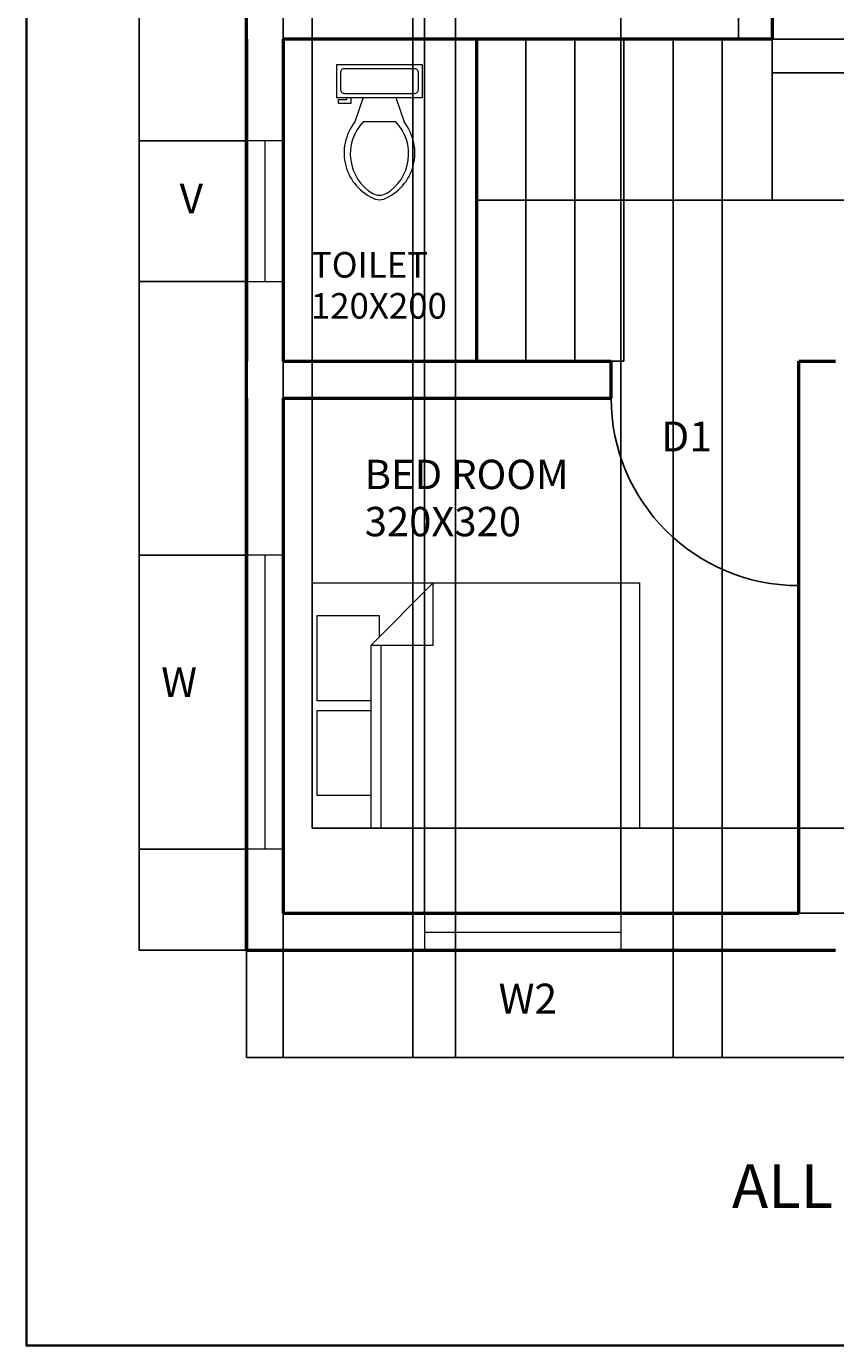
# Model space of a CAD drawing. Units: centimetres. Extents: x 2050 to 3144, y 831 to 2296.
# Tile 1 of 7: x 2050 to 2553, y 831 to 1650. Entities that reach past the tile are written whole.
import ezdxf

# ---------------------------------------------------------------- set-up
doc = ezdxf.new("R2010")
doc.units = ezdxf.units.CM
for name, color, linetype, lineweight in [('A-ANNO-DIMS', 2, 'Continuous', 18), ('A-ANNO-TEXT', 7, 'Continuous', 18), ('A-ANNO-TTLB', 7, 'Continuous', 35), ('A-AREA-IDEN', 7, 'Continuous', 25), ('A-DOOR', 3, 'Continuous', 25), ('A-FLOR-FIXT', 8, 'Continuous', 18), ('A-FLOR-STRS', 7, 'Continuous', 25), ('A-FURN', 8, 'Continuous', 18), ('A-GLAZ', 4, 'Continuous', 18), ('A-WALL', 7, 'Continuous', 50)]:
    doc.layers.add(name, color=color, linetype=linetype, lineweight=lineweight)
doc.styles.get("Standard").update_dxf_attribs({"font": 'arial.ttf'})
doc.dimstyles.get("Standard").update_dxf_attribs({"dimtxt": 0.18, "dimasz": 0.18, "dimexe": 0.18, "dimexo": 0.0625, "dimgap": 0.09, "dimtad": 0, "dimtih": 1, "dimtoh": 1, "dimdec": 4, "dimzin": 0, "dimdsep": 46, "dimtxsty": 'Standard', "dimcen": 0.09, "dimadec": 0, "dimazin": 0, "dimtfac": 1, "dimtdec": 4, "dimtofl": 0, "dimtmove": 0, "dimatfit": 3, "dimfxl": 1, "dimtolj": 1, "dimtzin": 0, "dimarcsym": 0})

# ---------------------------------------------------------------- blocks, each defined once
blk = doc.blocks.new('Toilet - top')
for p, q in [((9.5, -6), (9.5, -2)), ((-10, -8.5), (-8, -8.5)), ((-10, -9.5), (-10, -8.5)), ((-7, -9.5), (-10, -9.5)), ((-8, -8.5), (-8, -8)), ((-7, -8), (-7, -9.5)), ((-4, -8), (-6, -14)), ((4, -8), (6, -14)), ((4, -14), (-4, -14))]:
    blk.add_line(p, q)
blk.add_lwpolyline([(10.5, -8), (10.5, 0), (-10.5, 0), (-10.5, -8)], close=True)
for points in [[(-9.5, -2), (-9.5, -6)], [(8.5, -1), (-8.5, -1)], [(-8.5, -7), (8.5, -7)]]:
    blk.add_lwpolyline(points)
for centre, radius, start, end in [((-8.62, -1.88), 0.884, 81.8699, 188.1301), ((8.62, -1.88), 0.884, 351.8699, 98.1301), ((-8.62, -6.12), 0.884, 171.8699, 278.1301), ((8.62, -6.12), 0.884, 261.8699, 8.1301), ((3.52, -21.58), 12.17, 141.4691, 247.9714), ((4.2, -21.82), 11.33, 136.3677, 238.9468), ((-3.52, -21.58), 12.17, 292.0284, 38.5307), ((-4.2, -21.82), 11.33, 301.053, 43.6321), ((0, -27.88), 4, 245.7318, 294.2682), ((0, -29), 4, 254.8605, 285.1395)]:
    blk.add_arc(centre, radius, start, end)
blk = doc.blocks.new('Bed - Queen')
for p, q in [((0, -80.00003), (0, 0)), ((0, 0), (59.99999, 0)), ((59.99999, 0), (59.99999, -80.00003)), ((7.99999, -1.2), (28.79998, -1.2)), ((7.99999, -14.4), (7.99999, -1.2)), ((28.79998, -1.2), (28.79998, -14.4)), ((31.19999, -1.2), (51.99999, -1.2)), ((31.19999, -14.4), (31.19999, -1.2)), ((51.99999, -1.2), (51.99999, -16.4)), ((0, -14.4), (44.8, -14.4)), ((59.99999, -29.6), (44.8, -14.4)), ((44.8, -14.4), (44.8, -29.6)), ((44.8, -16.8), (0, -16.8)), ((51.99999, -16.4), (46.79936, -16.4)), ((44.8, -29.6), (59.99999, -29.6)), ((59.99999, -80.00003), (0, -80.00003))]:
    blk.add_line(p, q)
blk = doc.blocks.new('DOOR-D1-1165')
blk.add_line((116.51, 0), (116.51, 139.37))
blk.add_arc((116.51, 116.51), 116.51, 180, 270)
blk = doc.blocks.new('*D15')
at = {"layer": 'A-ANNO-DIMS', "color": 0, "lineweight": -2, "transparency": 16777216}
for p, q in [((2513.3, 1781.4), (2492.28, 1781.4)), ((2492.46, 1781.22), (2492.46, 1711.9)), ((2492.46, 1642.21), (2492.46, 1711.53)), ((2513.3, 1642.03), (2492.28, 1642.03))]:
    blk.add_line(p, q, dxfattribs=at)
at = {"layer": 'A-ANNO-DIMS', "color": 0, "transparency": 16777216}
for points in [[(2492.43, 1781.22), (2492.49, 1781.22), (2492.46, 1781.4)], [(2492.43, 1642.21), (2492.49, 1642.21), (2492.46, 1642.03)]]:
    blk.add_solid(points, dxfattribs=at)
at = {"layer": 'Defpoints', "color": 0, "transparency": 16777216}
for p in [(2513.36, 1781.4), (2492.46, 1642.03), (2513.36, 1642.03)]:
    blk.add_point(p, dxfattribs=at)
at = {"layer": 'A-ANNO-DIMS', "color": 0, "transparency": 16777216, "insert": (2492.46, 1711.72), "char_height": 0.18, "attachment_point": 5}
blk.add_mtext('\\A1;DOOR D1 139 TYP.', dxfattribs=at)
blk = doc.blocks.new('*D16')
at = {"layer": 'A-ANNO-DIMS', "color": 0, "lineweight": -2, "transparency": 16777216}
for p, q in [((2513.36, 1641.97), (2513.36, 1620.95)), ((2629.87, 1641.97), (2629.87, 1620.95)), ((2513.54, 1621.13), (2571.02, 1621.13)), ((2629.69, 1621.13), (2572.2, 1621.13))]:
    blk.add_line(p, q, dxfattribs=at)
at = {"layer": 'A-ANNO-DIMS', "color": 0, "transparency": 16777216}
for points in [[(2513.54, 1621.16), (2513.54, 1621.1), (2513.36, 1621.13)], [(2629.69, 1621.16), (2629.69, 1621.1), (2629.87, 1621.13)]]:
    blk.add_solid(points, dxfattribs=at)
at = {"layer": 'Defpoints', "color": 0, "transparency": 16777216}
for p in [(2513.36, 1642.03), (2629.87, 1642.03), (2629.87, 1621.13)]:
    blk.add_point(p, dxfattribs=at)
at = {"layer": 'A-ANNO-DIMS', "color": 0, "transparency": 16777216, "insert": (2571.61, 1621.13), "char_height": 0.18, "attachment_point": 5}
blk.add_mtext('\\A1;117 TYP.', dxfattribs=at)
blk = doc.blocks.new('*D31')
at = {"layer": 'A-ANNO-DIMS', "color": 0, "lineweight": -2, "transparency": 16777216}
for p, q in [((2187.01, 1076.25), (2187.01, 1009.53)), ((2975.59, 1076.25), (2975.59, 1009.53)), ((2187.19, 1009.71), (2580.9, 1009.71)), ((2975.41, 1009.71), (2581.69, 1009.71))]:
    blk.add_line(p, q, dxfattribs=at)
at = {"layer": 'A-ANNO-DIMS', "color": 0, "transparency": 16777216}
for points in [[(2187.19, 1009.74), (2187.19, 1009.68), (2187.01, 1009.71)], [(2975.41, 1009.74), (2975.41, 1009.68), (2975.59, 1009.71)]]:
    blk.add_solid(points, dxfattribs=at)
at = {"layer": 'Defpoints', "color": 0, "transparency": 16777216}
for p in [(2187.01, 1076.31), (2975.59, 1076.31), (2975.59, 1009.71)]:
    blk.add_point(p, dxfattribs=at)
at = {"layer": 'A-ANNO-DIMS', "color": 0, "transparency": 16777216, "insert": (2581.3, 1009.71), "char_height": 0.18, "attachment_point": 5}
blk.add_mtext('\\A1;788.6', dxfattribs=at)
blk = doc.blocks.new('*D32')
at = {"layer": 'A-ANNO-DIMS', "color": 0, "lineweight": -2, "transparency": 16777216}
for p, q in [((2186.94, 2087.75), (2120.23, 2087.75)), ((2120.41, 2087.57), (2120.41, 1582.22)), ((2120.41, 1076.49), (2120.41, 1581.85)), ((2186.94, 1076.31), (2120.23, 1076.31))]:
    blk.add_line(p, q, dxfattribs=at)
at = {"layer": 'A-ANNO-DIMS', "color": 0, "transparency": 16777216}
for points in [[(2120.38, 2087.57), (2120.44, 2087.57), (2120.41, 2087.75)], [(2120.38, 1076.49), (2120.44, 1076.49), (2120.41, 1076.31)]]:
    blk.add_solid(points, dxfattribs=at)
at = {"layer": 'Defpoints', "color": 0, "transparency": 16777216}
for p in [(2120.41, 2087.75), (2187.01, 2087.75), (2187.01, 1076.31)]:
    blk.add_point(p, dxfattribs=at)
at = {"layer": 'A-ANNO-DIMS', "color": 0, "transparency": 16777216, "insert": (2120.41, 1582.03), "char_height": 0.18, "attachment_point": 5}
blk.add_mtext('\\A1;1011.4', dxfattribs=at)
blk = doc.blocks.new('*D38')
at = {"layer": 'A-ANNO-DIMS', "color": 0, "lineweight": -2, "transparency": 16777216}
for p, q in [((2186.94, 1139.08), (2120.23, 1139.08)), ((2120.41, 1138.9), (2120.41, 1107.88)), ((2120.41, 1076.49), (2120.41, 1107.52)), ((2186.94, 1076.31), (2120.23, 1076.31))]:
    blk.add_line(p, q, dxfattribs=at)
at = {"layer": 'A-ANNO-DIMS', "color": 0, "transparency": 16777216}
for points in [[(2120.38, 1138.9), (2120.44, 1138.9), (2120.41, 1139.08)], [(2120.38, 1076.49), (2120.44, 1076.49), (2120.41, 1076.31)]]:
    blk.add_solid(points, dxfattribs=at)
at = {"layer": 'Defpoints', "color": 0, "transparency": 16777216}
for p in [(2120.41, 1139.08), (2187.01, 1139.08), (2187.01, 1076.31)]:
    blk.add_point(p, dxfattribs=at)
at = {"layer": 'A-ANNO-DIMS', "color": 0, "transparency": 16777216, "insert": (2120.41, 1107.7), "char_height": 0.18, "attachment_point": 5}
blk.add_mtext('\\A1;62.77', dxfattribs=at)
blk = doc.blocks.new('*D39')
at = {"layer": 'A-ANNO-DIMS', "color": 0, "lineweight": -2, "transparency": 16777216}
for p, q in [((2186.94, 1321.51), (2120.23, 1321.51)), ((2120.41, 1321.33), (2120.41, 1230.48)), ((2120.41, 1139.26), (2120.41, 1230.12)), ((2186.94, 1139.08), (2120.23, 1139.08))]:
    blk.add_line(p, q, dxfattribs=at)
at = {"layer": 'A-ANNO-DIMS', "color": 0, "transparency": 16777216}
for points in [[(2120.38, 1321.33), (2120.44, 1321.33), (2120.41, 1321.51)], [(2120.38, 1139.26), (2120.44, 1139.26), (2120.41, 1139.08)]]:
    blk.add_solid(points, dxfattribs=at)
at = {"layer": 'Defpoints', "color": 0, "transparency": 16777216}
for p in [(2120.41, 1321.51), (2187.01, 1321.51), (2187.01, 1139.08)]:
    blk.add_point(p, dxfattribs=at)
at = {"layer": 'A-ANNO-DIMS', "color": 0, "transparency": 16777216, "insert": (2120.41, 1230.3), "char_height": 0.18, "attachment_point": 5}
blk.add_mtext('\\A1;182.43', dxfattribs=at)
blk = doc.blocks.new('*D40')
at = {"layer": 'A-ANNO-DIMS', "color": 0, "lineweight": -2, "transparency": 16777216}
for p, q in [((2186.94, 1491.53), (2120.23, 1491.53)), ((2120.41, 1491.35), (2120.41, 1406.7)), ((2120.41, 1321.69), (2120.41, 1406.34)), ((2186.94, 1321.51), (2120.23, 1321.51))]:
    blk.add_line(p, q, dxfattribs=at)
at = {"layer": 'A-ANNO-DIMS', "color": 0, "transparency": 16777216}
for points in [[(2120.38, 1491.35), (2120.44, 1491.35), (2120.41, 1491.53)], [(2120.38, 1321.69), (2120.44, 1321.69), (2120.41, 1321.51)]]:
    blk.add_solid(points, dxfattribs=at)
at = {"layer": 'Defpoints', "color": 0, "transparency": 16777216}
for p in [(2120.41, 1491.53), (2187.01, 1491.53), (2187.01, 1321.51)]:
    blk.add_point(p, dxfattribs=at)
at = {"layer": 'A-ANNO-DIMS', "color": 0, "transparency": 16777216, "insert": (2120.41, 1406.52), "char_height": 0.18, "attachment_point": 5}
blk.add_mtext('\\A1;170.02', dxfattribs=at)
blk = doc.blocks.new('*D41')
at = {"layer": 'A-ANNO-DIMS', "color": 0, "lineweight": -2, "transparency": 16777216}
for p, q in [((2186.94, 1578.89), (2120.23, 1578.89)), ((2120.41, 1578.71), (2120.41, 1535.39)), ((2120.41, 1491.71), (2120.41, 1535.03)), ((2186.94, 1491.53), (2120.23, 1491.53))]:
    blk.add_line(p, q, dxfattribs=at)
at = {"layer": 'A-ANNO-DIMS', "color": 0, "transparency": 16777216}
for points in [[(2120.38, 1578.71), (2120.44, 1578.71), (2120.41, 1578.89)], [(2120.38, 1491.71), (2120.44, 1491.71), (2120.41, 1491.53)]]:
    blk.add_solid(points, dxfattribs=at)
at = {"layer": 'Defpoints', "color": 0, "transparency": 16777216}
for p in [(2120.41, 1578.89), (2187.01, 1578.89), (2187.01, 1491.53)]:
    blk.add_point(p, dxfattribs=at)
at = {"layer": 'A-ANNO-DIMS', "color": 0, "transparency": 16777216, "insert": (2120.41, 1535.21), "char_height": 0.18, "attachment_point": 5}
blk.add_mtext('\\A1;87.36', dxfattribs=at)
blk = doc.blocks.new('*D42')
at = {"layer": 'A-ANNO-DIMS', "color": 0, "lineweight": -2, "transparency": 16777216}
for p, q in [((2186.94, 1742.97), (2120.23, 1742.97)), ((2120.41, 1742.79), (2120.41, 1661.12)), ((2120.41, 1579.07), (2120.41, 1660.75)), ((2186.94, 1578.89), (2120.23, 1578.89))]:
    blk.add_line(p, q, dxfattribs=at)
at = {"layer": 'A-ANNO-DIMS', "color": 0, "transparency": 16777216}
for points in [[(2120.38, 1742.79), (2120.44, 1742.79), (2120.41, 1742.97)], [(2120.38, 1579.07), (2120.44, 1579.07), (2120.41, 1578.89)]]:
    blk.add_solid(points, dxfattribs=at)
at = {"layer": 'Defpoints', "color": 0, "transparency": 16777216}
for p in [(2120.41, 1742.97), (2187.01, 1742.97), (2187.01, 1578.89)]:
    blk.add_point(p, dxfattribs=at)
at = {"layer": 'A-ANNO-DIMS', "color": 0, "transparency": 16777216, "insert": (2120.41, 1660.93), "char_height": 0.18, "attachment_point": 5}
blk.add_mtext('\\A1;164.08', dxfattribs=at)
blk = doc.blocks.new('*D47')
at = {"layer": 'A-ANNO-DIMS', "color": 0, "lineweight": -2, "transparency": 16777216}
for p, q in [((2209.87, 1099.24), (2209.87, 2154.53)), ((2210.05, 2154.35), (2253.35, 2154.35)), ((2297.29, 2154.35), (2253.99, 2154.35)), ((2297.47, 1099.24), (2297.47, 2154.53))]:
    blk.add_line(p, q, dxfattribs=at)
at = {"layer": 'A-ANNO-DIMS', "color": 0, "transparency": 16777216}
for points in [[(2210.05, 2154.38), (2210.05, 2154.32), (2209.87, 2154.35)], [(2297.29, 2154.38), (2297.29, 2154.32), (2297.47, 2154.35)]]:
    blk.add_solid(points, dxfattribs=at)
at = {"layer": 'Defpoints', "color": 0, "transparency": 16777216}
for p in [(2297.47, 2154.35), (2209.87, 1099.17), (2297.47, 1099.17)]:
    blk.add_point(p, dxfattribs=at)
at = {"layer": 'A-ANNO-DIMS', "color": 0, "transparency": 16777216, "insert": (2253.67, 2154.35), "char_height": 0.18, "attachment_point": 5}
blk.add_mtext('\\A1;87.6', dxfattribs=at)
blk = doc.blocks.new('*D51')
at = {"layer": 'A-ANNO-DIMS', "color": 0, "lineweight": -2, "transparency": 16777216}
for p, q in [((2451.79, 1541.97), (2451.79, 1009.53)), ((2482.27, 1541.97), (2482.27, 1009.53)), ((2451.97, 1009.71), (2466.63, 1009.71)), ((2482.09, 1009.71), (2467.42, 1009.71))]:
    blk.add_line(p, q, dxfattribs=at)
at = {"layer": 'A-ANNO-DIMS', "color": 0, "transparency": 16777216}
for points in [[(2451.97, 1009.74), (2451.97, 1009.68), (2451.79, 1009.71)], [(2482.09, 1009.74), (2482.09, 1009.68), (2482.27, 1009.71)]]:
    blk.add_solid(points, dxfattribs=at)
at = {"layer": 'Defpoints', "color": 0, "transparency": 16777216}
for p in [(2451.79, 1542.03), (2482.27, 1542.03), (2482.27, 1009.71)]:
    blk.add_point(p, dxfattribs=at)
at = {"layer": 'A-ANNO-DIMS', "color": 0, "transparency": 16777216, "insert": (2467.03, 1009.71), "char_height": 0.18, "attachment_point": 5}
blk.add_mtext('\\A1;30.48', dxfattribs=at)
blk = doc.blocks.new('*D52')
at = {"layer": 'A-ANNO-DIMS', "color": 0, "lineweight": -2, "transparency": 16777216}
for p, q in [((2513.42, 1642.03), (3042.37, 1642.03)), ((3042.19, 1641.85), (3042.19, 1592.22)), ((3042.19, 1542.21), (3042.19, 1591.85)), ((2513.42, 1542.03), (3042.37, 1542.03))]:
    blk.add_line(p, q, dxfattribs=at)
at = {"layer": 'A-ANNO-DIMS', "color": 0, "transparency": 16777216}
for points in [[(3042.16, 1641.85), (3042.22, 1641.85), (3042.19, 1642.03)], [(3042.16, 1542.21), (3042.22, 1542.21), (3042.19, 1542.03)]]:
    blk.add_solid(points, dxfattribs=at)
at = {"layer": 'Defpoints', "color": 0, "transparency": 16777216}
for p in [(2513.36, 1642.03), (3042.19, 1642.03), (2513.36, 1542.03)]:
    blk.add_point(p, dxfattribs=at)
at = {"layer": 'A-ANNO-DIMS', "color": 0, "transparency": 16777216, "insert": (3042.19, 1592.03), "char_height": 0.18, "attachment_point": 5}
blk.add_mtext('\\A1;100', dxfattribs=at)
blk = doc.blocks.new('*D53')
at = {"layer": 'A-ANNO-DIMS', "color": 0, "lineweight": -2, "transparency": 16777216}
for p, q in [((2209.87, 1664.83), (2209.87, 1009.53)), ((2290.25, 1664.83), (2290.25, 1009.53)), ((2210.05, 1009.71), (2249.67, 1009.71)), ((2290.07, 1009.71), (2250.45, 1009.71))]:
    blk.add_line(p, q, dxfattribs=at)
at = {"layer": 'A-ANNO-DIMS', "color": 0, "transparency": 16777216}
for points in [[(2210.05, 1009.74), (2210.05, 1009.68), (2209.87, 1009.71)], [(2290.07, 1009.74), (2290.07, 1009.68), (2290.25, 1009.71)]]:
    blk.add_solid(points, dxfattribs=at)
at = {"layer": 'Defpoints', "color": 0, "transparency": 16777216}
for p in [(2209.87, 1664.89), (2290.25, 1664.89), (2290.25, 1009.71)]:
    blk.add_point(p, dxfattribs=at)
at = {"layer": 'A-ANNO-DIMS', "color": 0, "transparency": 16777216, "insert": (2250.06, 1009.71), "char_height": 0.18, "attachment_point": 5}
blk.add_mtext('\\A1;80.39', dxfattribs=at)
blk = doc.blocks.new('*D63')
at = {"layer": 'A-ANNO-DIMS', "color": 0, "lineweight": -2, "transparency": 16777216}
for p, q in [((2297.47, 1099.24), (2297.47, 2154.53)), ((2297.65, 2154.35), (2357.98, 2154.35)), ((2419.21, 2154.35), (2358.89, 2154.35)), ((2419.39, 1099.24), (2419.39, 2154.53))]:
    blk.add_line(p, q, dxfattribs=at)
at = {"layer": 'A-ANNO-DIMS', "color": 0, "transparency": 16777216}
for points in [[(2297.65, 2154.38), (2297.65, 2154.32), (2297.47, 2154.35)], [(2419.21, 2154.38), (2419.21, 2154.32), (2419.39, 2154.35)]]:
    blk.add_solid(points, dxfattribs=at)
at = {"layer": 'Defpoints', "color": 0, "transparency": 16777216}
for p in [(2419.39, 2154.35), (2297.47, 1099.17), (2419.39, 1099.17)]:
    blk.add_point(p, dxfattribs=at)
at = {"layer": 'A-ANNO-DIMS', "color": 0, "transparency": 16777216, "insert": (2358.43, 2154.35), "char_height": 0.18, "attachment_point": 5}
blk.add_mtext('\\A1;121.92', dxfattribs=at)
blk = doc.blocks.new('*D66')
at = {"layer": 'A-ANNO-DIMS', "color": 0, "lineweight": -2, "transparency": 16777216}
for p, q in [((2209.87, 1139.14), (2209.87, 2154.53)), ((2210.05, 2154.35), (2218.38, 2154.35)), ((2227.62, 2154.35), (2219.29, 2154.35)), ((2227.8, 1152.03), (2227.8, 2154.53))]:
    blk.add_line(p, q, dxfattribs=at)
at = {"layer": 'A-ANNO-DIMS', "color": 0, "transparency": 16777216}
for points in [[(2210.05, 2154.38), (2210.05, 2154.32), (2209.87, 2154.35)], [(2227.62, 2154.38), (2227.62, 2154.32), (2227.8, 2154.35)]]:
    blk.add_solid(points, dxfattribs=at)
at = {"layer": 'Defpoints', "color": 0, "transparency": 16777216}
for p in [(2227.8, 2154.35), (2227.8, 1151.97), (2209.87, 1139.08)]:
    blk.add_point(p, dxfattribs=at)
at = {"layer": 'A-ANNO-DIMS', "color": 0, "transparency": 16777216, "insert": (2218.83, 2154.35), "char_height": 0.18, "attachment_point": 5}
blk.add_mtext('\\A1;17.933', dxfattribs=at)
blk = doc.blocks.new('*D67')
at = {"layer": 'A-ANNO-DIMS', "color": 0, "lineweight": -2, "transparency": 16777216}
for p, q in [((2227.86, 1151.97), (3042.37, 1151.97)), ((3042.19, 1151.79), (3042.19, 1125.75)), ((3042.19, 1099.35), (3042.19, 1125.39)), ((2209.93, 1099.17), (3042.37, 1099.17))]:
    blk.add_line(p, q, dxfattribs=at)
at = {"layer": 'A-ANNO-DIMS', "color": 0, "transparency": 16777216}
for points in [[(3042.16, 1151.79), (3042.22, 1151.79), (3042.19, 1151.97)], [(3042.16, 1099.35), (3042.22, 1099.35), (3042.19, 1099.17)]]:
    blk.add_solid(points, dxfattribs=at)
at = {"layer": 'Defpoints', "color": 0, "transparency": 16777216}
for p in [(2227.8, 1151.97), (2209.87, 1099.17), (3042.19, 1099.17)]:
    blk.add_point(p, dxfattribs=at)
at = {"layer": 'A-ANNO-DIMS', "color": 0, "transparency": 16777216, "insert": (3042.19, 1125.57), "char_height": 0.18, "attachment_point": 5}
blk.add_mtext('\\A1;52.79', dxfattribs=at)
blk = doc.blocks.new('*D70')
at = {"layer": 'A-ANNO-DIMS', "color": 0, "lineweight": -2, "transparency": 16777216}
for p, q in [((2209.87, 2064.83), (2209.87, 1009.53)), ((2316.84, 2059.23), (2316.84, 1009.53)), ((2210.05, 1009.71), (2262.9, 1009.71)), ((2316.66, 1009.71), (2263.81, 1009.71))]:
    blk.add_line(p, q, dxfattribs=at)
at = {"layer": 'A-ANNO-DIMS', "color": 0, "transparency": 16777216}
for points in [[(2210.05, 1009.74), (2210.05, 1009.68), (2209.87, 1009.71)], [(2316.66, 1009.74), (2316.66, 1009.68), (2316.84, 1009.71)]]:
    blk.add_solid(points, dxfattribs=at)
at = {"layer": 'Defpoints', "color": 0, "transparency": 16777216}
for p in [(2209.87, 2064.89), (2316.84, 2059.29), (2316.84, 1009.71)]:
    blk.add_point(p, dxfattribs=at)
at = {"layer": 'A-ANNO-DIMS', "color": 0, "transparency": 16777216, "insert": (2263.35, 1009.71), "char_height": 0.18, "attachment_point": 5}
blk.add_mtext('\\A1;106.97', dxfattribs=at)

msp = doc.modelspace()

# ---------------------------------------------------------------- linework, layer by layer
at = {"layer": 'A-ANNO-TTLB'}
msp.add_lwpolyline([(2050.3641, 2295.8578), (3143.7558, 2295.8578), (3143.7558, 830.6902), (2050.3641, 830.6902)], close=True, dxfattribs=at)
at = {"layer": 'A-FLOR-STRS'}
for p, q in [((2360.3465, 1642.0348), (2360.3465, 1442.0348)), ((2390.8265, 1642.0348), (2390.8265, 1442.0348)), ((2421.3065, 1642.0348), (2421.3065, 1442.0348)), ((2451.7865, 1642.0348), (2451.7865, 1542.0348)), ((2482.2665, 1642.0348), (2482.2665, 1542.0348)), ((2513.3612, 1642.0348), (2513.3612, 1542.0348)), ((2513.3612, 1542.0348), (2329.8665, 1542.0348)), ((2413.3612, 1442.0348), (2421.3065, 1442.0348))]:
    msp.add_line(p, q, dxfattribs=at)
at = {"layer": 'A-GLAZ'}
for p, q in [((2209.8665, 1578.8921), (2187.0065, 1578.8921)), ((2198.4365, 1578.8921), (2198.4365, 1491.5301)), ((2187.0065, 1491.5301), (2209.8665, 1491.5301)), ((2209.8665, 1321.513), (2187.0065, 1321.513)), ((2198.4365, 1321.513), (2198.4365, 1139.0811)), ((2209.8665, 1139.0811), (2187.0065, 1139.0811)), ((2297.4733, 1099.1748), (2297.4733, 1076.3148)), ((2419.3933, 1099.1748), (2419.3933, 1076.3148)), ((2297.4733, 1087.4723), (2419.3933, 1087.4723))]:
    msp.add_line(p, q, dxfattribs=at)
at = {"layer": 'A-WALL'}
for p, q in [((2187.0065, 1076.3148), (2187.0065, 2087.7548)), ((2513.3612, 1664.8948), (2513.3612, 1642.0348)), ((2187.0065, 1642.0348), (2187.0065, 1442.0348)), ((2209.8665, 1642.0348), (2209.8665, 1442.0348)), ((2513.3612, 1642.0348), (2209.8665, 1642.0348)), ((2329.8665, 1642.0348), (2329.8665, 1442.0348)), ((2209.8665, 1442.0348), (2413.3612, 1442.0348)), ((2413.3612, 1419.1748), (2413.3612, 1442.0348)), ((2529.8665, 1099.1748), (2529.8665, 1442.0348)), ((2529.8665, 1442.0348), (2552.7265, 1442.0348)), ((2187.0065, 1419.1748), (2187.0065, 1076.3148)), ((2209.8665, 1419.1748), (2413.3612, 1419.1748)), ((2209.8665, 1419.1748), (2209.8665, 1099.1748)), ((2209.8665, 1099.1748), (2529.8665, 1099.1748)), ((2187.0065, 1076.3148), (2552.7265, 1076.3148))]:
    msp.add_line(p, q, dxfattribs=at)

# ---------------------------------------------------------------- block references
at = {"layer": 'A-DOOR', "extrusion": (0, 0, -1), "zscale": -1, "rotation": 180}
msp.add_blockref('DOOR-D1-1165', (-2513.361, 1781.4006), dxfattribs=at)
at = {"layer": 'A-DOOR'}
msp.add_blockref('DOOR-D1-1165', (2413.361, 1302.669), dxfattribs=at)
at = {"layer": 'A-FLOR-FIXT', "xscale": 2.54, "yscale": 2.54, "zscale": 2.54}
msp.add_blockref('Toilet - top', (2269.5685, 1626.163), dxfattribs=at)
at = {"layer": 'A-FURN', "xscale": 2.54, "yscale": 2.54, "zscale": 2.54, "rotation": 90}
msp.add_blockref('Bed - Queen', (2227.7996, 1151.9671), dxfattribs=at)

# ---------------------------------------------------------------- texts
at = {"layer": 'A-ANNO-TEXT'}
for s, height, p in [('V', 18.5959, (2145.4428, 1533.7818)), ('D1', 18.59595, (2444.4269, 1385.9903)), ('W', 18.5959, (2134.0485, 1233.4159)), ('W2', 18.59595, (2343.4962, 1036.8754)), ('ALL DIMENSION IN CENTIMETER', 27.192544, (2488.3592, 916.1363))]:
    msp.add_text(s, height=height, dxfattribs=at).set_placement(p)
at = {"layer": 'A-AREA-IDEN'}
for s, height, p in [('TOILET', 15.8597, (2226.9643, 1493.9662)), ('120X200', 15.8597, (2226.9643, 1468.489)), ('BED ROOM', 18.23402, (2260.3697, 1362.6011)), ('320X320', 18.23402, (2260.3697, 1333.3098))]:
    msp.add_text(s, height=height, dxfattribs=at).set_placement(p)

# ---------------------------------------------------------------- dimensions: what is measured, and where the dimension line sits
at = {"layer": 'A-ANNO-DIMS'}
for base, p1, p2, override, picture, middle in [((2297.4733, 2154.3548), (2209.8665, 1099.1748), (2297.4733, 1099.1748), {"dimdec": 1, "dimlfac": 1, "dimrnd": 0, "dimzin": 0, "dimdsep": 46, "dimlunit": 2}, '*D47', (2253.6699, 2154.3548)), ((2227.7996, 2154.3548), (2209.8665, 1139.0811), (2227.7996, 1151.9671), {"dimdec": 3, "dimlfac": 1, "dimrnd": 0, "dimzin": 0, "dimdsep": 46, "dimlunit": 2}, '*D66', (2218.8331, 2154.3548)), ((2419.3933, 2154.3548), (2297.4733, 1099.1748), (2419.3933, 1099.1748), {"dimdec": 2, "dimlfac": 1, "dimrnd": 0, "dimzin": 0, "dimdsep": 46, "dimlunit": 2}, '*D63', (2358.4333, 2154.3548)), ((2316.8368, 1009.7148), (2209.8665, 2064.8948), (2316.8368, 2059.2924), {"dimdec": 2, "dimlfac": 1, "dimrnd": 0, "dimzin": 0, "dimdsep": 46, "dimlunit": 2}, '*D70', (2263.3517, 1009.7148)), ((2290.2526, 1009.7148), (2209.8665, 1664.8948), (2290.2526, 1664.8948), {"dimdec": 2, "dimlfac": 1, "dimrnd": 0, "dimzin": 0, "dimdsep": 46, "dimlunit": 2}, '*D53', (2250.0596, 1009.7148)), ((2482.2665, 1009.7148), (2451.7865, 1542.0348), (2482.2665, 1542.0348), {"dimdec": 2, "dimlfac": 1, "dimrnd": 0, "dimzin": 0, "dimdsep": 46, "dimlunit": 2}, '*D51', (2467.0265, 1009.7148)), ((2975.5865, 1009.7148), (2187.0065, 1076.3148), (2975.5865, 1076.3148), {"dimdec": 1, "dimlfac": 1, "dimrnd": 0, "dimzin": 0, "dimdsep": 46, "dimlunit": 2}, '*D31', (2581.2965, 1009.7148))]:
    dim = msp.add_linear_dim(base=base, p1=p1, p2=p2, dimstyle='Standard', override=override, dxfattribs=at)
    dim.commit()
    dim.dimension.update_dxf_attribs({"geometry": picture, "text_midpoint": middle})
for base, p1, p2, override, picture, middle in [((2120.4065, 2087.7548), (2187.0065, 1076.3148), (2187.0065, 2087.7548), {"dimdec": 1, "dimlfac": 1, "dimrnd": 0, "dimzin": 0, "dimdsep": 46, "dimlunit": 2}, '*D32', (2120.4065, 1582.0348)), ((2120.4065, 1742.9748), (2187.0065, 1578.8921), (2187.0065, 1742.9748), {"dimdec": 2, "dimlfac": 1, "dimrnd": 0, "dimzin": 0, "dimdsep": 46, "dimlunit": 2}, '*D42', (2120.4065, 1660.9335)), ((3042.1865, 1642.0348), (2513.3612, 1542.0348), (2513.3612, 1642.0348), {"dimdec": 0, "dimlfac": 1, "dimrnd": 0, "dimzin": 0, "dimdsep": 46, "dimlunit": 2}, '*D52', (3042.1865, 1592.0348)), ((2120.4065, 1578.8921), (2187.0065, 1491.5301), (2187.0065, 1578.8921), {"dimdec": 2, "dimlfac": 1, "dimrnd": 0, "dimzin": 0, "dimdsep": 46, "dimlunit": 2}, '*D41', (2120.4065, 1535.2111)), ((2120.4065, 1491.5301), (2187.0065, 1321.513), (2187.0065, 1491.5301), {"dimdec": 2, "dimlfac": 1, "dimrnd": 0, "dimzin": 0, "dimdsep": 46, "dimlunit": 2}, '*D40', (2120.4065, 1406.5216)), ((2120.4065, 1321.513), (2187.0065, 1139.0811), (2187.0065, 1321.513), {"dimdec": 2, "dimlfac": 1, "dimrnd": 0, "dimzin": 0, "dimdsep": 46, "dimlunit": 2}, '*D39', (2120.4065, 1230.2971)), ((3042.1865, 1099.1748), (2227.7996, 1151.9671), (2209.8665, 1099.1748), {"dimdec": 2, "dimlfac": 1, "dimrnd": 0, "dimzin": 0, "dimdsep": 46, "dimlunit": 2}, '*D67', (3042.1865, 1125.5709)), ((2120.4065, 1139.0811), (2187.0065, 1076.3148), (2187.0065, 1139.0811), {"dimdec": 2, "dimlfac": 1, "dimrnd": 0, "dimzin": 0, "dimdsep": 46, "dimlunit": 2}, '*D38', (2120.4065, 1107.6979))]:
    dim = msp.add_linear_dim(base=base, p1=p1, p2=p2, angle=90, dimstyle='Standard', override=override, dxfattribs=at)
    dim.commit()
    dim.dimension.update_dxf_attribs({"geometry": picture, "text_midpoint": middle})
dim = msp.add_linear_dim(base=(2492.4564, 1642.0348), p1=(2513.3612, 1781.4001), p2=(2513.3612, 1642.0348), angle=270, text='DOOR D1 <> TYP.', dimstyle='Standard', override={"dimdec": 0, "dimlfac": 1, "dimrnd": 0, "dimzin": 0, "dimdsep": 46, "dimlunit": 2}, dxfattribs=at)
dim.commit()
dim.dimension.update_dxf_attribs({"geometry": '*D15', "text_midpoint": (2492.4564, 1711.7175)})
dim = msp.add_linear_dim(base=(2629.8665, 1621.13), p1=(2513.3612, 1642.0348), p2=(2629.8665, 1642.0348), text='<> TYP.', dimstyle='Standard', override={"dimdec": 0, "dimlfac": 1, "dimrnd": 0, "dimzin": 0, "dimdsep": 46, "dimlunit": 2}, dxfattribs=at)
dim.commit()
dim.dimension.update_dxf_attribs({"geometry": '*D16', "text_midpoint": (2571.6139, 1621.13)})

doc.saveas('drawing.dxf')
